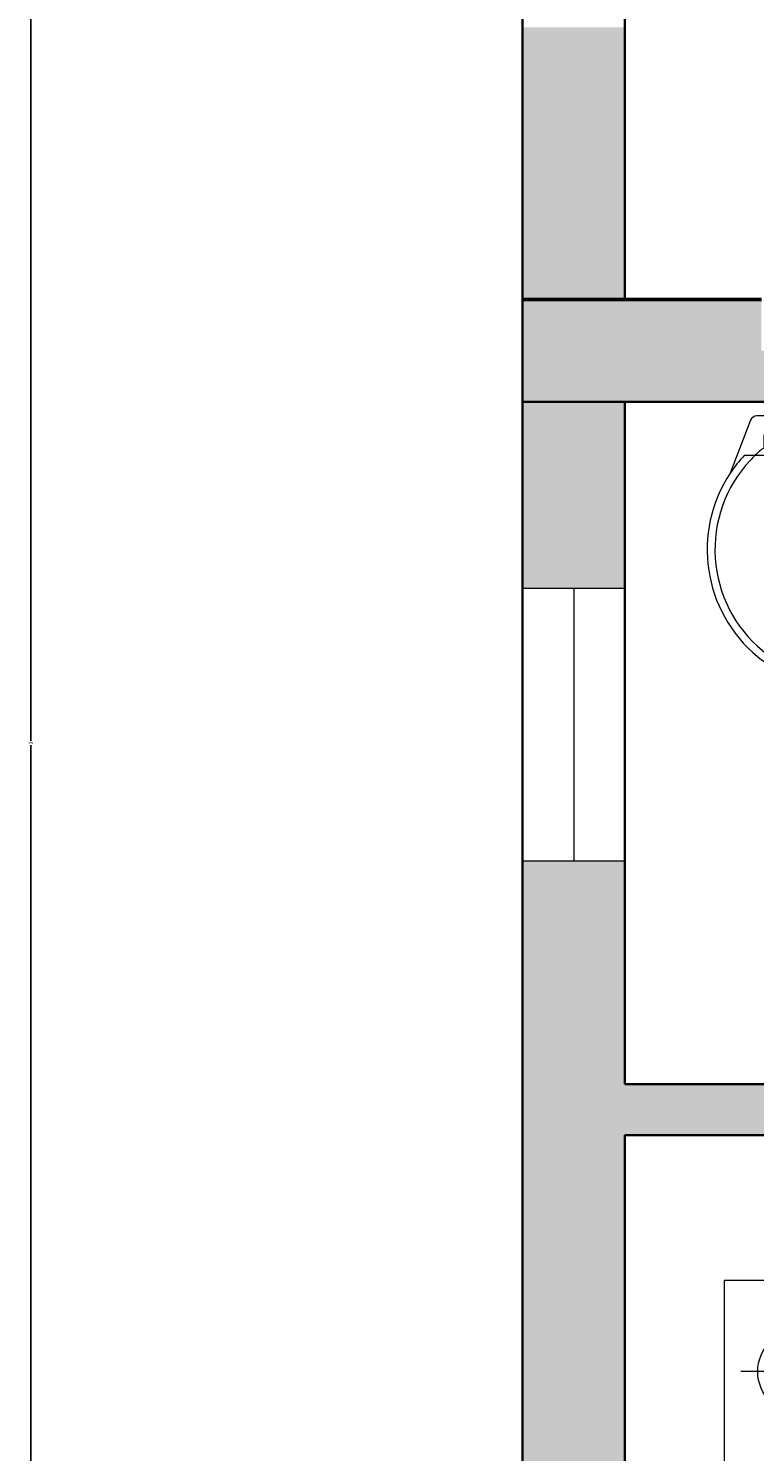
# Model space of a CAD drawing. Units: inches. Extents: x -28 to 485, y -861 to 54.
# Tile 7 of 14: x -28 to 36, y -240 to -115. Entities that reach past the tile are written whole.
import ezdxf

# ---------------------------------------------------------------- set-up
doc = ezdxf.new("R2010")
doc.units = ezdxf.units.IN
doc.header["$MEASUREMENT"] = 0
for name, color, linetype, lineweight in [('A-ANNO-DIMS', 2, 'Continuous', 18), ('A-COLS', 7, 'Continuous', 50), ('A-COLS-PATT', 8, 'Continuous', 13), ('A-FLOR-FIXT', 9, 'Continuous', 18), ('A-FURN', 8, 'Continuous', 13), ('A-GLAZ', 4, 'Continuous', 18), ('A-WALL', 7, 'Continuous', 35), ('A-WALL-PATT', 34, 'Continuous', 13)]:
    doc.layers.add(name, color=color, linetype=linetype, lineweight=lineweight)
doc.styles.get("Standard").update_dxf_attribs({"font": 'arial.ttf'})
doc.dimstyles.get("Standard").update_dxf_attribs({"dimtxt": 0.18, "dimasz": 0.18, "dimexe": 0.18, "dimexo": 0.0625, "dimgap": 0.09, "dimtad": 0, "dimtih": 1, "dimtoh": 1, "dimdec": 0, "dimzin": 0, "dimdsep": 46, "dimlunit": 3, "dimtxsty": 'Standard', "dimcen": 0.09, "dimadec": 0, "dimazin": 0, "dimtfac": 1, "dimtdec": 0, "dimtofl": 0, "dimtmove": 0, "dimatfit": 3, "dimfxl": 1, "dimtolj": 1, "dimtzin": 0, "dimarcsym": 0})

# ---------------------------------------------------------------- blocks, each defined once
blk = doc.blocks.new('BED-DOUBLE-WITH-NIGHTSTANDS')
for p, q in [((0, 0), (0, 80.08)), ((6.67, 66.84), (6.67, 77.31)), ((11.91, 72.08), (1.44, 72.08)), ((39.26, 64.51), (39.26, 68.96)), ((39.26, 68.96), (68.11, 68.96)), ((68.11, 68.96), (68.11, 10.57)), ((40.19, 68.03), (40.19, 64.5)), ((67.18, 68.03), (40.19, 68.03)), ((67.18, 11.5), (67.18, 68.03)), ((1.03, 64.07), (1.03, 16.02)), ((12.66, 16.02), (12.66, 64.07)), ((15.98, 63.85), (16.38, 35.34)), ((44.25, 64.43), (44.25, 15.09)), ((45.25, 64.51), (45.25, 15.09)), ((16.8, 63.82), (17.22, 34.74)), ((19.33, 63.78), (19.45, 33.37)), ((20.15, 63.78), (20.27, 33.06)), ((59.06, 60.14), (58.15, 60.31)), ((53.12, 56.3), (53.12, 23.78)), ((59.06, 54.54), (58.15, 54.36)), ((12.66, 38.02), (18.76, 33.63)), ((15.04, 27.14), (12.66, 35.87)), ((18.76, 33.63), (23.47, 31.84)), ((23.47, 31.84), (25.57, 31.52)), ((25.57, 31.52), (24.92, 28.93)), ((24.92, 28.93), (23.95, 26.82)), ((17.14, 21.3), (15.04, 27.14)), ((23.95, 26.82), (23.47, 23.25)), ((59.06, 24.99), (58.15, 25.16)), ((23.47, 23.25), (23.14, 19.19)), ((19.41, 18.22), (17.14, 21.3)), ((23.14, 19.19), (23.47, 15.95)), ((59.06, 19.39), (58.15, 19.21)), ((22.82, 15.3), (19.41, 18.22)), ((0, 16.02), (21.98, 16.02)), ((23.47, 15.95), (22.82, 15.3)), ((39.26, 10.57), (39.26, 15.1)), ((40.19, 15.1), (40.19, 11.5)), ((6.67, 13.24), (6.67, 2.78)), ((40.19, 11.5), (67.18, 11.5)), ((68.11, 10.57), (39.26, 10.57)), ((11.91, 8.01), (1.44, 8.01))]:
    blk.add_line(p, q)
for points in [[(0, 64.07), (13.35, 64.07), (13.35, 80.08), (0, 80.08)], [(6.67, 72.08), (5.06, 71.14)], [(6.67, 72.08), (8.29, 71.14)], [(13.35, 16.02), (13.35, 0), (0, 0)], [(6.67, 8.01), (5.06, 8.94)], [(6.67, 8.01), (8.29, 8.94)]]:
    blk.add_lwpolyline(points)
for points in [[(43.62, 64.41, 0.056112), (48.03, 64.99, 0.095341), (52.27, 66.12)], [(2, 59.47, -0.074897), (7.23, 59.37, 0.472817)], [(7.52, 43.09, -0.14099), (2.18, 42.93, -0.235245)], [(7.52, 39.67, 0.14099), (2.18, 39.83, 0.235245)], [(2, 20.62, 0.074897), (7.23, 20.71, -0.472817)], [(30.15, 15.13, 0.001242), (45.35, 15.09, -0.127202), (52.92, 13.49)]]:
    blk.add_lwpolyline(points, format="xyb")
for centre, radius in [((6.67, 72.08), 3.74), ((6.67, 72.08), 1.87), ((64.11, 56.84), 0.204), ((61.96, 55.51), 0.204), ((61.96, 24.02), 0.204), ((64.11, 22.68), 0.204), ((6.67, 8.01), 3.74), ((6.67, 8.01), 1.87)]:
    blk.add_circle(centre, radius)
for centre, radius, start, end in [((69.62, 57.92), 10.46, 111.4092, 145.6135), ((68.59, 75.81), 10.46, 228.1144, 262.255), ((69.99, 70.57), 5.1, 209.8884, 236.5383), ((70.94, 72.4), 6.35, 223.5186, 233.6964), ((52.68, 65.51), 0.73, 336.5219, 123.8264), ((131.01, 58.75), 77.93, 175.2402, 181.8035), ((22.44, 207.63), 143.9, 266.1, 270.9282), ((27.68, 251.44), 187.71, 269.1145, 274.8735), ((60.79, 62.99), 0.867, 76.272, 177.0484), ((61.24, 62.69), 1.16, 20.9613, 102.2885), ((68.81, 67.71), 4.25, 221.0454, 247.4453), ((66.52, 79.36), 14.47, 266.3481, 272.5919), ((58.76, 65.61), 6.06, 203.6453, 236.3329), ((55.85, 62.08), 1.35, 88.9462, 185.5144), ((56.04, 61.53), 1.91, 7.1143, 95.0551), ((59.12, 61.97), 1.2, 19.1312, 189.736), ((60.43, 62.21), 0.737, 126.7319, 206.0245), ((59.47, 64.76), 1.79, 284.7031, 328.6173), ((61.96, 62.49), 1.65, 125.7657, 194.5347), ((53.85, 65.41), 7.32, 332.8176, 347.4827), ((61.86, 63.85), 0.873, 181.7131, 301.5367), ((59, 62.09), 2.64, 2.0648, 41.1598), ((60.59, 63.07), 0.856, 316.2238, 62.3173), ((61.09, 62.57), 0.0682, 20.2667, 316.2271), ((56.85, 62.5), 2.41, 193.079, 274.7067), ((55.32, 60.77), 1.86, 338.5779, 68.4181), ((55.62, 61.86), 2.33, 305.9599, 357.6409), ((56.48, 64.35), 3.78, 288.2955, 328.7386), ((58.76, 62.26), 1.5, 285.6955, 4.031), ((60.76, 60.64), 1.6, 128.4175, 173.8338), ((61.51, 62.18), 0.13, 168.5166, 2.0648), ((61.45, 62.19), 0.0631, 52.0591, 168.5166), ((53.71, 63.39), 3.32, 259.249, 301.1782), ((55.15, 57.49), 3.09, 85.2696, 124.215), ((57.33, 61.13), 1.99, 196.8663, 330.0915), ((55.15, 57.49), 3.09, 53.6555, 57.2989), ((56.78, 64.39), 4.3, 273.4924, 303.7117), ((-760.15, 15.33), 763.42, 2.85022, 3.31479), ((9.33, 49.26), 10.32, 78.2417, 114.8684), ((1.06, 56.61), 10.73, 348.9631, 14.8961), ((54, 59.28), 0.964, 127.675, 162.5814), ((54, 59.28), 0.964, 196.6343, 225.5483), ((54.57, 60.82), 2.55, 240.8249, 340.7178), ((53.81, 59.69), 1.2, 246.1646, 318.4347), ((55.03, 61.2), 2.3, 240.0851, 262.564), ((55.94, 57.8), 1.64, 74.8529, 138.4347), ((56.5, 59.87), 0.497, 254.8529, 12.6959), ((60.19, 59.12), 0.158, 125.0752, 284.7644), ((60.43, 59.18), 0.34, 127.3642, 168.4363), ((60.17, 59.45), 0.49, 277.4968, 341.2737), ((60.56, 59.22), 0.195, 88.1325, 178.8919), ((60.95, 59.02), 0.422, 136.3462, 189.6513), ((60.71, 58.98), 0.176, 189.6513, 312.3208), ((60.75, 59.46), 0.204, 183.2768, 356.7232), ((61.39, 59.1), 0.668, 164.2829, 186.9148), ((60.6, 59.09), 0.334, 312.3208, 40.2111), ((61.31, 59.47), 0.474, 201.6382, 274.947), ((60.68, 58.82), 0.619, 42.3896, 66.5724), ((66.93, 63.72), 7.6, 217.9541, 226.8459), ((61.13, 59.18), 0.337, 10.9597, 52.2379), ((61.33, 59.15), 0.156, 274.947, 37.5263), ((62.33, 58.47), 0.42, 115.5379, 168.6744), ((60.9, 59.07), 1.27, 329.344, 349.7412), ((59.89, 58.78), 2.26, 352.8698, 1.6736), ((61.28, 51.56), 6.63, 110.1059, 116.9968), ((59.01, 57.53), 0.163, 83.9457, 185.6216), ((58.36, 57.69), 0.671, 328.836, 0.8141), ((58.71, 57.49), 0.384, 306.5232, 32.4668), ((59.16, 57.79), 0.163, 112.5583, 214.2343), ((59.06, 58.08), 0.384, 265.7131, 351.6568), ((58.72, 58.29), 0.671, 297.3659, 329.344), ((58.21, 58.87), 1.29, 313.6929, 321.7899), ((59.64, 57.99), 0.42, 115.5379, 168.6744), ((58.21, 58.6), 1.27, 329.344, 349.7412), ((61.28, 51.56), 6.63, 86.1723, 106.4158), ((57.2, 58.31), 2.26, 352.8698, 1.6736), ((61.86, 58.27), 0.163, 112.5583, 214.2343), ((61.75, 58.56), 0.384, 265.7131, 351.6568), ((61.42, 58.77), 0.671, 297.3659, 329.344), ((61.45, 54.86), 3.33, 60.7959, 85.244), ((54.37, 50.07), 10.94, 37.8256, 47.7588), ((60.91, 59.35), 1.29, 313.6929, 321.7899), ((63.07, 58.33), 0.228, 33.0979, 123.1364), ((58.05, 55.12), 5.96, 31.1156, 34.8118), ((62.74, 57.94), 0.617, 2.3172, 70.5201), ((62.44, 57.27), 0.93, 310.9365, 22.7695), ((63.25, 57.78), 0.178, 135.7354, 318.1297), ((62.95, 58.07), 0.236, 315.7354, 31.1156), ((62.75, 57.57), 0.547, 319.3812, 5.5456), ((63.38, 57.79), 0.178, 68.2452, 250.6395), ((62.97, 58), 0.531, 352.6008, 57.1845), ((64.87, 54.44), 3.55, 111.7087, 116.2181), ((61.45, 54.86), 3.33, 47.5083, 55.9967), ((63.48, 58.12), 0.531, 252.8042, 349.6943), ((62.97, 57.17), 0.565, 331.1838, 51.6792), ((63.53, 58.17), 0.236, 248.2452, 323.6254), ((63.33, 58.31), 0.617, 291.7087, 3.0299), ((58.93, 61.56), 5.96, 323.6254, 327.3216), ((63.81, 58.16), 0.228, 325.6077, 55.6462), ((54.57, 53.85), 2.55, 19.2822, 119.1751), ((57.16, 57.12), 0.251, 169.5864, 349.5616), ((57.25, 57.11), 0.154, 349.5616, 167.2949), ((59.06, 57.02), 0.42, 129.5056, 182.6421), ((57.85, 58), 1.27, 308.4388, 328.836), ((57.63, 59.02), 2.26, 296.5064, 305.3102), ((57.61, 57.86), 1.29, 336.3901, 344.4871), ((61.66, 57.07), 0.93, 253.6301, 325.4631), ((61.92, 55.78), 0.658, 82.0748, 142.6895), ((61.87, 56.57), 0.565, 273.8774, 357.1501), ((62.09, 56.97), 0.547, 262.0748, 308.2393), ((62.97, 56.41), 0.565, 181.4625, 249.4747), ((62.87, 56.86), 0.547, 215.1128, 261.2773), ((63.31, 56.83), 0.93, 197.889, 269.722), ((65.87, 54.52), 3.99, 130.182, 149.456), ((63.67, 56.79), 0.658, 139.3812, 199.9959), ((62.87, 57.22), 0.675, 285.6484, 332.2957), ((63.55, 56.5), 0.158, 125.0752, 284.7644), ((63.8, 56.56), 0.34, 93.635, 168.4363), ((63.75, 57.1), 0.2, 138.2946, 276.2474), ((63.53, 56.83), 0.49, 277.4968, 341.2737), ((63.83, 57.07), 0.278, 358.5719, 143.8954), ((63.92, 56.61), 0.195, 88.1325, 178.8919), ((63.99, 57.29), 0.281, 208.8493, 269.9355), ((63.75, 57.22), 0.321, 274.2123, 318.1587), ((64.31, 56.4), 0.422, 136.3462, 189.6513), ((64.75, 56.48), 0.668, 164.2829, 186.9148), ((64.73, 56.9), 0.643, 121.9501, 165.2442), ((63.96, 56.47), 0.334, 312.3208, 40.2111), ((64.67, 56.85), 0.474, 201.6382, 274.947), ((64.28, 57.14), 0.135, 262.868, 7.094), ((64.04, 56.2), 0.619, 42.3896, 66.5724), ((64.27, 57.26), 0.403, 278.5614, 22.5914), ((64.49, 56.56), 0.337, 10.9597, 118.7804), ((64.49, 57.27), 0.202, 44.3732, 121.9501), ((64.7, 56.53), 0.156, 274.947, 37.5263), ((54, 55.39), 0.964, 134.4517, 156.7144), ((53.81, 54.99), 1.2, 41.5653, 113.8354), ((55.03, 53.47), 2.3, 97.436, 119.9149), ((55.94, 56.87), 1.64, 221.5653, 285.1471), ((57.33, 53.55), 1.99, 29.9085, 163.1337), ((56.5, 54.81), 0.497, 347.3041, 105.1471), ((61.4, 55.17), 0.158, 125.0752, 284.7644), ((61.65, 55.23), 0.34, 93.635, 168.4363), ((61.85, 56.68), 0.675, 228.342, 274.9894), ((61.6, 55.76), 0.2, 138.2946, 276.2474), ((61.38, 55.5), 0.49, 277.4968, 341.2737), ((61.68, 55.73), 0.278, 358.5719, 143.8954), ((61.77, 55.27), 0.195, 88.1325, 178.8919), ((61.84, 55.95), 0.281, 208.8493, 269.9355), ((61.6, 55.89), 0.321, 274.2123, 318.1587), ((62.16, 55.06), 0.422, 136.3462, 189.6513), ((62.6, 55.14), 0.668, 164.2829, 186.9148), ((62.58, 55.56), 0.643, 121.9501, 165.2442), ((61.81, 55.14), 0.334, 312.3208, 40.2111), ((62.52, 55.52), 0.474, 201.6382, 274.947), ((62.13, 55.81), 0.135, 262.868, 7.094), ((61.89, 54.87), 0.619, 42.3896, 66.5724), ((62.12, 55.92), 0.403, 278.5614, 22.5914), ((62.34, 55.23), 0.337, 10.9597, 118.7804), ((65.87, 54.52), 3.99, 156.1523, 156.9499), ((62.34, 55.94), 0.202, 44.3732, 121.9501), ((62.55, 55.2), 0.156, 274.947, 37.5263), ((63.02, 56.51), 0.675, 248.3627, 295.0101), ((62.69, 55.67), 0.658, 20.6625, 81.2773), ((64.07, 56.36), 0.176, 189.6513, 312.3208), ((1.85, 51.98), 10.19, 333.8761, 16.1746), ((54, 55.39), 0.964, 203.2856, 232.325), ((53.71, 51.28), 3.32, 58.8218, 100.2867), ((58.76, 49.06), 6.06, 123.6671, 158.5059), ((55.15, 57.18), 3.09, 235.785, 274.7304), ((56.85, 52.18), 2.41, 85.2933, 166.921), ((55.32, 53.9), 1.86, 291.5819, 21.4221), ((55.15, 57.18), 3.09, 302.7011, 306.3445), ((55.62, 52.81), 2.33, 2.3591, 54.0401), ((56.78, 50.29), 4.3, 56.2883, 86.5076), ((56.48, 50.32), 3.78, 31.2614, 71.7045), ((60.76, 54.03), 1.6, 186.1662, 231.5825), ((58.76, 52.42), 1.5, 355.969, 74.3045), ((61.92, 55.02), 0.176, 189.6513, 312.3208), ((65.87, 54.52), 3.99, 175.2415, 182.8929), ((16.01, 49.96), 14.08, 166.3427, 191.1841), ((55.85, 52.59), 1.35, 174.4856, 271.0538), ((56.04, 53.15), 1.91, 264.9449, 352.8857), ((59.12, 52.71), 1.2, 170.264, 340.8688), ((60.43, 52.46), 0.737, 153.9755, 233.2681), ((61.96, 52.19), 1.65, 165.4653, 234.2343), ((53.85, 49.26), 7.32, 12.5173, 27.1824), ((61.51, 52.5), 0.13, 357.9352, 191.4834), ((60.79, 51.69), 0.867, 182.9516, 283.728), ((59.47, 49.92), 1.79, 31.3827, 75.2969), ((59, 52.59), 2.64, 318.8402, 357.9352), ((60.59, 51.6), 0.856, 297.6827, 43.7762), ((61.86, 50.82), 0.873, 58.4633, 178.2869), ((61.24, 51.98), 1.16, 257.7115, 339.0387), ((61.13, 52.12), 0.113, 43.7762, 339.7183), ((61.45, 52.48), 0.0631, 191.4834, 307.9409), ((69.62, 56.75), 10.46, 214.3865, 248.5908), ((68.81, 46.96), 4.25, 112.5547, 138.9546), ((66.17, 41.19), 8.09, 82.8636, 171.8197), ((66.52, 35.31), 14.47, 87.4081, 93.6519), ((66.74, 46.53), 1.88, 76.3898, 169.0739), ((74.19, 42.33), 10.46, 152.5854, 175.5377), ((66.48, 45.12), 2.37, 72.8609, 131.9049), ((65.43, 42.24), 4.68, 68.117, 96.6195), ((72.68, 45.26), 5.75, 162.9798, 196.4569), ((5.99, 44.03), 3.96, 153.3437, 196.1026), ((7.37, 44.56), 4.25, 335.0183, 18.5407), ((75.64, 42.98), 8.5, 174.3643, 175.6213), ((10.2, 52.53), 9.81, 254.1707, 275.9871), ((58.94, 41.49), 1.16, 50.8855, 132.2127), ((64.01, 42.31), 0.867, 106.1963, 206.9726), ((61.98, 43.19), 1.79, 314.6273, 358.5415), ((65.27, 42.46), 1.65, 155.6899, 224.4589), ((64.54, 42.29), 1.16, 50.8855, 132.2127), ((64.51, 43.6), 0.873, 211.6373, 331.4609), ((63.8, 42.29), 0.856, 346.148, 92.2415), ((62.91, 40.64), 2.64, 31.989, 71.0841), ((56.78, 40.96), 7.32, 2.7418, 17.407), ((81.47, 38.5), 15.2, 160.0972, 160.2783), ((58.4, 41.51), 0.867, 106.1963, 206.9726), ((56.38, 42.39), 1.79, 314.6273, 358.5415), ((59.67, 41.66), 1.65, 155.6899, 224.4589), ((59.67, 40.53), 1.65, 135.5411, 204.3101), ((58.91, 42.8), 0.873, 211.6373, 331.4609), ((58.2, 41.49), 0.856, 346.148, 92.2415), ((57.3, 39.84), 2.64, 31.989, 71.0841), ((51.18, 40.16), 7.32, 2.7418, 17.407), ((51.18, 42.04), 7.32, 342.593, 357.2582), ((58.87, 41.3), 0.0682, 50.1909, 346.0209), ((64.47, 42.1), 0.0682, 50.1909, 346.0209), ((64.98, 41.95), 0.0631, 81.9833, 198.4408), ((65.04, 41.98), 0.13, 198.4408, 31.989), ((58.4, 40.68), 0.867, 153.0274, 253.8037), ((56.38, 39.81), 1.79, 1.4585, 45.3727), ((57.3, 42.35), 2.64, 288.9159, 328.011), ((58.2, 40.71), 0.856, 267.7585, 13.852), ((58.91, 39.39), 0.873, 28.5391, 148.3627), ((58.92, 40.88), 0.113, 13.852, 309.9245), ((59.44, 41.17), 0.13, 198.4408, 31.989), ((59.37, 41.15), 0.0631, 81.9833, 198.4408), ((59.44, 41.02), 0.13, 328.011, 161.5592), ((59.37, 41.04), 0.0631, 161.5592, 278.0167), ((64.01, 39.88), 0.867, 153.0274, 253.8037), ((61.98, 39.01), 1.79, 1.4585, 45.3727), ((65.27, 39.73), 1.65, 135.5411, 204.3101), ((56.78, 41.24), 7.32, 342.593, 357.2582), ((62.91, 41.55), 2.64, 288.9159, 328.011), ((63.8, 39.91), 0.856, 267.7585, 13.852), ((64.52, 40.08), 0.113, 13.852, 309.9245), ((64.98, 40.24), 0.0631, 161.5592, 278.0167), ((65.04, 40.22), 0.13, 328.011, 161.5592), ((16.3, 37.72), 14.27, 171.5249, 193.96), ((10.2, 30.23), 9.81, 84.0129, 105.8293), ((-2.51, 36.66), 14.12, 349.8617, 13.6238), ((58.94, 40.71), 1.16, 227.7873, 309.1145), ((68.59, 40.66), 10.46, 184.4623, 262.255), ((64.51, 38.59), 0.873, 28.5391, 148.3627), ((64.54, 39.91), 1.16, 227.7873, 309.1145), ((74.19, 39.86), 10.46, 184.4623, 207.4146), ((72.68, 36.94), 5.75, 163.5431, 197.0202), ((75.64, 39.22), 8.5, 184.3787, 185.6357), ((81.47, 43.7), 15.2, 199.7217, 199.9028), ((30.98, 31.59), 29.04, 172.2196, 189.497), ((-6.57, 29.12), 18.61, 348.0397, 19.2615), ((69.99, 35.42), 5.1, 181.272, 236.5383), ((72.72, 40.59), 9.45, 214.0123, 234.053), ((70.94, 37.25), 6.35, 197.8504, 233.6964), ((-4.69, 37.08), 31.06, 340.1194, 349.3383), ((25.64, 31.34), 0.193, 358.8623, 109.7536), ((69.62, 22.77), 10.46, 111.4092, 145.6135), ((66.52, 44.21), 14.47, 266.3481, 272.5919), ((68.81, 32.56), 4.25, 221.0454, 247.4453), ((58.76, 30.46), 6.06, 201.4941, 236.3329), ((55.85, 26.93), 1.35, 88.9462, 185.5144), ((56.04, 26.38), 1.91, 7.1143, 95.0551), ((59.12, 26.82), 1.2, 19.1312, 189.736), ((60.43, 27.07), 0.737, 126.7319, 206.0245), ((60.79, 27.84), 0.867, 76.272, 177.0484), ((59.47, 29.61), 1.79, 284.7031, 328.6173), ((61.96, 27.34), 1.65, 125.7657, 194.5347), ((53.85, 30.27), 7.32, 332.8176, 347.4827), ((61.24, 27.55), 1.16, 20.9613, 102.2885), ((60.59, 27.92), 0.856, 316.2238, 62.3173), ((59, 26.94), 2.64, 2.0648, 41.1598), ((61.86, 28.71), 0.873, 181.7131, 301.5367), ((-760.15, 64.76), 763.42, 356.68521, 357.14978), ((30.48, 23.89), 6.52, 156.2616, 191.3392), ((56.85, 27.35), 2.41, 193.079, 274.7067), ((55.32, 25.63), 1.86, 338.5779, 68.4181), ((55.62, 26.71), 2.33, 305.9599, 357.6409), ((56.48, 29.2), 3.78, 288.2955, 328.7386), ((58.76, 27.11), 1.5, 285.6955, 4.031), ((60.76, 25.49), 1.6, 128.4175, 173.8338), ((61.09, 27.42), 0.0682, 20.2667, 316.2271), ((61.51, 27.03), 0.13, 168.5166, 2.0648), ((61.45, 27.04), 0.0631, 52.0591, 168.5166), ((1.06, 23.47), 10.73, 345.1039, 11.0369), ((53.71, 28.24), 3.32, 259.7133, 301.1782), ((55.15, 22.34), 3.09, 85.2696, 124.215), ((57.33, 25.98), 1.99, 196.8663, 330.0915), ((56.78, 29.24), 4.3, 273.4924, 303.7117), ((65.87, 25.01), 3.99, 177.1071, 184.7585), ((136.48, 22.83), 83.37, 179.3433, 185.6887), ((54, 24.13), 0.964, 127.675, 156.7144), ((54.57, 25.67), 2.55, 240.8249, 340.7178), ((55.03, 26.06), 2.3, 240.0851, 262.564), ((55.94, 22.65), 1.64, 74.8529, 138.4347), ((56.5, 24.72), 0.497, 254.8529, 12.6959), ((55.15, 22.34), 3.09, 53.6555, 57.2989), ((61.4, 24.36), 0.158, 75.2356, 234.9248), ((61.65, 24.3), 0.34, 191.5637, 266.365), ((61.6, 23.76), 0.2, 83.7526, 221.7054), ((61.38, 24.03), 0.49, 18.7263, 82.5032), ((61.68, 23.79), 0.278, 216.1046, 1.4281), ((61.77, 24.25), 0.195, 181.1081, 271.8675), ((61.84, 23.57), 0.281, 90.0645, 151.1507), ((61.6, 23.64), 0.321, 41.8413, 85.7877), ((61.92, 24.5), 0.176, 47.6792, 170.3487), ((62.16, 24.46), 0.422, 170.3487, 223.6538), ((62.6, 24.38), 0.668, 173.0852, 195.7171), ((62.58, 23.96), 0.643, 194.7558, 238.0499), ((61.81, 24.39), 0.334, 319.7889, 47.6792), ((62.52, 24.01), 0.474, 85.053, 158.3618), ((62.13, 23.71), 0.135, 352.906, 97.132), ((61.89, 24.66), 0.619, 293.4276, 317.6104), ((62.34, 24.29), 0.337, 241.2196, 349.0403), ((62.12, 23.6), 0.403, 337.4086, 81.4386), ((62.55, 24.33), 0.156, 322.4737, 85.053), ((-5.54, 16.67), 30.23, 357.4519, 11.3392), ((54, 24.13), 0.964, 203.229, 225.5483), ((53.81, 24.54), 1.2, 246.1646, 318.4347), ((57.16, 22.4), 0.251, 10.4384, 190.4136), ((61.85, 22.84), 0.675, 85.0106, 131.658), ((61.66, 22.46), 0.93, 34.5369, 106.3699), ((61.92, 23.75), 0.658, 217.3105, 277.9252), ((54.37, 29.45), 10.94, 312.2412, 322.1744), ((61.87, 22.95), 0.565, 2.8499, 86.1226), ((62.09, 22.55), 0.547, 51.7607, 97.9252), ((65.87, 25.01), 3.99, 203.0501, 203.8477), ((62.34, 23.59), 0.202, 238.0499, 315.6268), ((62.97, 23.11), 0.565, 110.5253, 178.5375), ((63.31, 22.7), 0.93, 90.278, 162.111), ((62.87, 22.67), 0.547, 98.7227, 144.8872), ((65.87, 25.01), 3.99, 210.544, 229.818), ((63.02, 23.01), 0.675, 64.9899, 111.6373), ((62.69, 23.86), 0.658, 278.7227, 339.3375), ((63.67, 22.74), 0.658, 160.0041, 220.6188), ((62.44, 22.26), 0.93, 337.2305, 49.0635), ((62.87, 22.31), 0.675, 27.7043, 74.3516), ((62.97, 22.35), 0.565, 308.3208, 28.8162), ((63.55, 23.03), 0.158, 75.2356, 234.9248), ((63.8, 22.96), 0.34, 191.5637, 266.365), ((63.75, 22.43), 0.2, 83.7526, 221.7054), ((63.53, 22.69), 0.49, 18.7263, 82.5032), ((63.92, 22.92), 0.195, 181.1081, 271.8675), ((63.75, 22.31), 0.321, 41.8413, 85.7877), ((64.07, 23.17), 0.176, 47.6792, 170.3487), ((64.31, 23.13), 0.422, 170.3487, 223.6538), ((64.75, 23.05), 0.668, 173.0852, 195.7171), ((63.96, 23.05), 0.334, 319.7889, 47.6792), ((64.67, 22.68), 0.474, 85.053, 158.3618), ((64.04, 23.32), 0.619, 293.4276, 317.6104), ((64.49, 22.96), 0.337, 241.2196, 349.0403), ((64.27, 22.27), 0.403, 337.4086, 81.4386), ((64.7, 22.99), 0.156, 322.4737, 85.053), ((9.33, 30.82), 10.32, 245.1316, 281.7583), ((57.25, 22.42), 0.154, 192.7051, 10.4384), ((61.28, 27.97), 6.63, 243.0032, 249.8941), ((57.85, 21.53), 1.27, 31.164, 51.5612), ((59.06, 22.5), 0.42, 177.3579, 230.4944), ((57.63, 20.5), 2.26, 54.6898, 63.4936), ((57.61, 21.66), 1.29, 15.5129, 23.6099), ((59.01, 21.99), 0.163, 174.3784, 276.0543), ((58.71, 22.03), 0.384, 327.5332, 53.4768), ((58.36, 21.84), 0.671, 359.1859, 31.164), ((59.16, 21.74), 0.163, 145.7657, 247.4417), ((59.06, 21.45), 0.384, 8.3432, 94.2869), ((58.72, 21.23), 0.671, 30.656, 62.6341), ((58.21, 20.66), 1.29, 38.2101, 46.3071), ((59.64, 21.53), 0.42, 191.3256, 244.4621), ((58.21, 20.93), 1.27, 10.2588, 30.656), ((61.28, 27.97), 6.63, 253.5842, 273.8277), ((57.2, 21.22), 2.26, 358.3264, 7.1302), ((66.93, 15.8), 7.6, 133.1541, 142.0459), ((61.86, 21.26), 0.163, 145.7657, 247.4417), ((61.45, 24.67), 3.33, 274.756, 299.2041), ((61.75, 20.97), 0.384, 8.3432, 94.2869), ((61.42, 20.76), 0.671, 30.656, 62.6341), ((62.74, 21.59), 0.617, 289.4799, 357.6828), ((58.05, 24.41), 5.96, 325.1882, 328.8844), ((63.25, 21.74), 0.178, 41.8703, 224.2646), ((62.95, 21.45), 0.236, 328.8844, 44.2646), ((62.75, 21.95), 0.547, 354.4544, 40.6188), ((63.38, 21.74), 0.178, 109.3605, 291.7548), ((62.97, 21.52), 0.531, 302.8155, 7.3992), ((64.87, 25.09), 3.55, 243.7819, 248.2913), ((61.45, 24.67), 3.33, 304.0033, 312.4917), ((63.48, 21.4), 0.531, 10.3057, 107.1958), ((63.53, 21.36), 0.236, 36.3746, 111.7548), ((63.33, 21.21), 0.617, 356.9701, 68.2913), ((63.83, 22.46), 0.278, 216.1046, 1.4281), ((58.93, 17.96), 5.96, 32.6784, 36.3746), ((63.99, 22.24), 0.281, 90.0645, 151.1507), ((63.81, 21.37), 0.228, 304.3538, 34.3923), ((64.73, 22.63), 0.643, 194.7558, 238.0499), ((64.28, 22.38), 0.135, 352.906, 97.132), ((64.49, 22.25), 0.202, 238.0499, 315.6268), ((54, 20.25), 0.964, 134.4517, 153.558), ((54.57, 18.71), 2.55, 19.2822, 119.1751), ((53.81, 19.84), 1.2, 41.5653, 113.8354), ((55.03, 18.32), 2.3, 97.436, 119.9149), ((55.94, 21.72), 1.64, 221.5653, 285.1471), ((57.33, 18.4), 1.99, 29.9085, 163.1337), ((56.5, 19.66), 0.497, 347.3041, 105.1471), ((60.19, 20.41), 0.158, 75.2356, 234.9248), ((60.43, 20.35), 0.34, 191.5637, 232.6358), ((60.17, 20.07), 0.49, 18.7263, 82.5032), ((60.56, 20.3), 0.195, 181.1081, 271.8675), ((60.71, 20.55), 0.176, 47.6792, 170.3487), ((60.95, 20.51), 0.422, 170.3487, 223.6538), ((60.75, 20.06), 0.204, 3.2768, 176.7232), ((61.39, 20.43), 0.668, 173.0852, 195.7171), ((60.6, 20.43), 0.334, 319.7889, 47.6792), ((61.31, 20.06), 0.474, 85.053, 158.3618), ((60.68, 20.7), 0.619, 293.4276, 317.6104), ((61.13, 20.34), 0.337, 307.7621, 349.0403), ((61.33, 20.37), 0.156, 322.4737, 85.053), ((60.91, 20.18), 1.29, 38.2101, 46.3071), ((62.33, 21.06), 0.42, 191.3256, 244.4621), ((60.9, 20.45), 1.27, 10.2588, 30.656), ((59.89, 20.74), 2.26, 358.3264, 7.1302), ((63.07, 21.2), 0.228, 236.8636, 326.9021), ((54, 20.25), 0.964, 210.0293, 232.325), ((53.71, 16.14), 3.32, 58.8218, 99.1554), ((58.76, 13.91), 6.06, 123.6671, 153.2997), ((55.15, 22.04), 3.09, 235.785, 274.7304), ((56.85, 17.03), 2.41, 85.2933, 166.921), ((55.32, 18.75), 1.86, 291.5819, 21.4221), ((55.15, 22.04), 3.09, 302.7011, 306.3445), ((55.62, 17.67), 2.33, 2.3591, 54.0401), ((56.78, 15.14), 4.3, 56.2883, 86.5076), ((55.85, 17.44), 1.35, 174.4856, 271.0538), ((56.04, 18), 1.91, 264.9449, 352.8857), ((56.48, 15.18), 3.78, 31.2614, 71.7045), ((59.12, 17.56), 1.2, 170.264, 340.8688), ((58.76, 17.27), 1.5, 355.969, 74.3045), ((60.76, 18.89), 1.6, 186.1662, 231.5825), ((60.43, 17.31), 0.737, 153.9755, 233.2681), ((59.47, 14.77), 1.79, 31.3827, 75.2969), ((60.79, 16.54), 0.867, 182.9516, 283.728), ((61.96, 17.04), 1.65, 165.4653, 234.2343), ((53.85, 14.11), 7.32, 12.5173, 27.1824), ((59, 17.44), 2.64, 318.8402, 357.9352), ((60.59, 16.46), 0.856, 297.6827, 43.7762), ((61.86, 15.67), 0.873, 58.4633, 178.2869), ((61.24, 16.83), 1.16, 257.7115, 339.0387), ((61.13, 16.97), 0.113, 43.7762, 339.7183), ((61.51, 17.35), 0.13, 357.9352, 191.4834), ((61.45, 17.33), 0.0631, 191.4834, 307.9409), ((24.81, -58.13), 73.46, 85.8294, 91.553), ((69.62, 21.6), 10.46, 214.3865, 248.5908), ((68.81, 11.81), 4.25, 112.5547, 138.9546), ((52.87, 14.23), 0.739, 273.98, 27.3412), ((68.59, 3.71), 10.46, 97.745, 131.8856), ((66.52, 0.17), 14.47, 87.4081, 93.6519), ((69.99, 8.96), 5.1, 123.4617, 150.1116), ((70.94, 7.13), 6.35, 126.3036, 136.4814)]:
    blk.add_arc(centre, radius, start, end)
blk = doc.blocks.new('WC-FLOOR-MOUNTED')
for p, q in [((3.27, 19.35), (4.23, 19.35)), ((4.23, 19.35), (8.71, 19.35)), ((13.2, 19.35), (8.71, 19.35)), ((13.2, 19.35), (14.16, 19.35))]:
    blk.add_line(p, q)
for points in [[(8.71, 22.81), (4.36, 22.81, 0.31031), (3.82, 22.44), (2.03, 17.79, 0.209071)], [(8.71, 22.81), (13.07, 22.81, -0.31031), (13.6, 22.44), (15.39, 17.79, -0.209071)], [(5.01, 20.04), (5.01, 21, -1), (6.47, 21), (6.47, 20.5)], [(12.41, 20.04), (12.41, 21, 1), (10.96, 21), (10.96, 20.5)], [(5.01, 20.04, 0.022712), (4.23, 19.35, 0.162618)], [(8.71, 20.04), (5.01, 20.04, 0.022712)], [(8.71, 20.04), (12.41, 20.04, -0.476108)], [(12.41, 20.04, -0.022712), (13.2, 19.35, -0.162618)], [(3.77, 18.89, 0.431639), (4.86, 2.17, 0.162618), (8.71, 0.68, 0.470877)], [(3.27, 19.35, 0.040937), (2.03, 17.79, 0.163732)], [(4.23, 19.35, 0.014165), (3.77, 18.89, 0.162618)], [(13.2, 19.35, -0.448546), (12.57, 2.17, -0.162618), (8.71, 0.68, -0.470877)], [(14.16, 19.35, -0.040937), (15.39, 17.79, -0.163732)], [(2.03, 17.79, 0.383919), (4.43, 1.64, 0.163732), (8.71, 0, 0.359733)], [(15.39, 17.79, -0.383919), (13, 1.64, -0.163732), (8.71, 0, -0.359733)]]:
    blk.add_lwpolyline(points, format="xyb")
for points in [[(10.96, 20.5), (6.47, 20.5)], [(6.47, 20.5), (6.47, 20.04)], [(10.96, 20.5), (10.96, 20.04)]]:
    blk.add_lwpolyline(points)
blk = doc.blocks.new('WINDOW-24IN')
for p, q in [((0, 24), (0, 0)), ((9, 24), (0, 24)), ((4.5, 24), (4.5, 0)), ((9, 0), (9, 24)), ((9, 0), (0, 0))]:
    blk.add_line(p, q)
blk = doc.blocks.new('*D54')
at = {"layer": 'A-ANNO-DIMS', "color": 0, "lineweight": -2, "transparency": 16777216}
for p, q in [((15.22, 10.13), (-28.15, 10.13)), ((-27.97, 9.95), (-27.97, -177.18)), ((-27.97, -364.69), (-27.97, -177.55)), ((15.22, -364.87), (-28.15, -364.87))]:
    blk.add_line(p, q, dxfattribs=at)
at = {"layer": 'A-ANNO-DIMS', "color": 0, "transparency": 16777216}
for points in [[(-28, 9.95), (-27.94, 9.95), (-27.97, 10.13)], [(-28, -364.69), (-27.94, -364.69), (-27.97, -364.87)]]:
    blk.add_solid(points, dxfattribs=at)
at = {"layer": 'Defpoints', "color": 0, "transparency": 16777216}
for p in [(15.28, 10.13), (-27.97, -364.87), (15.28, -364.87)]:
    blk.add_point(p, dxfattribs=at)
at = {"layer": 'A-ANNO-DIMS', "color": 0, "transparency": 16777216, "insert": (-27.97, -177.37), "char_height": 0.18, "attachment_point": 5}
blk.add_mtext('\\A1;375', dxfattribs=at)

msp = doc.modelspace()

# ---------------------------------------------------------------- hatches: boundary and pattern name
at = {"layer": 'A-COLS-PATT'}
h = msp.add_hatch(color=256, dxfattribs=at)
h.dxf.hatch_style = 1
h.paths.add_polyline_path([(36.285, 10.133), (15.285, 10.133), (15.285, 1.133), (36.285, 1.133)])
h.paths.add_polyline_path([(160.785, 10.133), (139.785, 10.133), (139.785, 1.133), (160.785, 1.133)])
h.paths.add_polyline_path([(316.785, 10.133), (295.785, 10.133), (295.785, 1.133), (316.785, 1.133)])
h.paths.add_polyline_path([(441.285, 10.133), (420.285, 10.133), (420.285, 1.133), (441.285, 1.133)])
h.paths.add_polyline_path([(441.285, -138.367), (432.285, -138.367), (420.285, -138.367), (420.285, -147.367), (441.285, -147.367)])
h.paths.add_polyline_path([(304.785, -130.867), (295.785, -130.867), (295.785, -147.367), (304.785, -147.367), (304.785, -142.867)])
h.paths.add_polyline_path([(160.785, -130.867), (151.785, -130.867), (151.785, -142.867), (151.785, -147.367), (160.785, -147.367)])
h.paths.add_polyline_path([(36.285, -138.367), (24.285, -138.367), (15.285, -138.367), (15.285, -147.367), (36.285, -147.367)])
h.paths.add_polyline_path([(36.285, -355.867), (15.285, -355.867), (15.285, -364.867), (36.285, -364.867)])
h.paths.add_polyline_path([(160.785, -355.867), (139.785, -355.867), (139.785, -364.867), (160.785, -364.867)])
h.paths.add_polyline_path([(316.785, -355.867), (300.285, -355.867), (295.785, -355.867), (295.785, -364.867), (316.785, -364.867)])
at = {"layer": 'A-WALL-PATT'}
h = msp.add_hatch(color=256, dxfattribs=at)
h.dxf.hatch_style = 1
h.paths.add_polyline_path([(160.785, -808.867), (160.785, -817.867), (295.785, -817.867), (295.785, -808.867)])
h.paths.add_polyline_path([(316.785, -817.867), (323.776, -817.867), (323.776, -808.867), (316.785, -808.867)])
h.paths.add_polyline_path([(420.285, -817.867), (420.285, -808.867), (383.776, -808.867), (383.776, -817.867)])
h.paths.add_polyline_path([(432.285, -808.867), (441.285, -808.867), (441.285, -702.966), (432.285, -702.966), (432.285, -708.367), (397.785, -708.367), (397.785, -710.617), (397.785, -712.867), (432.285, -712.867)])
h.paths.add_polyline_path([(300.285, -712.867), (329.285, -712.867), (329.285, -710.617), (329.285, -708.367), (295.785, -708.367), (295.785, -808.867), (300.285, -808.867)])
h.paths.add_polyline_path([(160.785, -698.867), (158.535, -698.867), (156.285, -698.867), (156.285, -808.867), (160.785, -808.867)])
h.paths.add_polyline_path([(36.285, -808.867), (36.285, -817.867), (79.721, -817.867), (79.721, -808.867)])
h.paths.add_polyline_path([(15.285, -808.867), (24.285, -808.867), (24.285, -739.09), (15.285, -739.09)])
h.paths.add_polyline_path([(24.285, -640.781), (15.285, -640.781), (15.285, -679.09), (24.285, -679.09), (24.285, -664.867), (89.285, -664.867), (89.285, -662.617), (89.285, -660.367), (24.285, -660.367)])
h.paths.add_polyline_path([(15.285, -616.781), (24.285, -616.781), (24.285, -600.367), (15.285, -600.367)])
h.paths.add_polyline_path([(36.285, -595.867), (36.285, -600.367), (123.285, -600.367), (123.285, -660.367), (117.285, -660.367), (117.285, -664.867), (156.285, -664.867), (156.285, -670.867), (160.785, -670.867), (160.785, -660.367), (127.785, -660.367), (127.785, -600.367), (129.785, -600.367), (129.785, -598.117), (129.785, -595.867)])
h.paths.add_polyline_path([(367.785, -664.867), (363.285, -664.867), (363.285, -708.367), (357.285, -708.367), (357.285, -712.867), (369.785, -712.867), (369.785, -708.367), (367.785, -708.367)])
h.paths.add_polyline_path([(432.285, -664.867), (432.285, -666.966), (441.285, -666.966), (441.285, -642.367), (432.285, -642.367), (432.285, -660.367), (328.785, -660.367), (328.785, -664.867), (363.285, -664.867)])
h.paths.add_polyline_path([(333.285, -600.367), (420.285, -600.367), (420.285, -595.867), (326.785, -595.867), (326.785, -600.367), (328.785, -600.367), (328.785, -630.367), (331.035, -630.367), (333.285, -630.367)])
h.paths.add_polyline_path([(441.285, -600.367), (432.285, -600.367), (432.285, -618.367), (441.285, -618.367)])
h.paths.add_polyline_path([(432.285, -591.367), (441.285, -591.367), (441.285, -547.793), (432.285, -547.793)])
h.paths.add_polyline_path([(295.785, -588.367), (300.238, -588.367), (300.285, -583.867), (300.285, -451.867), (295.785, -451.867)])
h.paths.add_polyline_path([(420.285, -451.867), (420.285, -442.867), (316.785, -442.867), (316.785, -451.867)])
h.paths.add_polyline_path([(432.285, -487.793), (441.285, -487.793), (441.285, -451.867), (432.285, -451.867)])
h.paths.add_polyline_path([(432.285, -442.867), (441.285, -442.867), (441.285, -364.867), (432.285, -364.867)])
h.paths.add_polyline_path([(261.785, -451.867), (261.785, -447.367), (261.785, -444.758), (261.785, -442.867), (160.785, -442.867), (160.785, -451.867)])
h.paths.add_polyline_path([(139.785, -451.867), (139.785, -442.867), (36.285, -442.867), (36.285, -451.867)])
h.paths.add_polyline_path([(15.285, -491.617), (24.285, -491.617), (24.285, -451.867), (15.285, -451.867)])
h.paths.add_polyline_path([(24.285, -551.617), (15.285, -551.617), (15.285, -591.367), (24.285, -591.367)])
h.paths.add_polyline_path([(160.785, -451.867), (156.285, -451.867), (156.285, -588.367), (160.785, -588.367)])
h.paths.add_polyline_path([(139.785, -364.867), (139.785, -355.867), (36.285, -355.867), (36.285, -364.867)])
h.paths.add_polyline_path([(24.285, -364.867), (15.285, -364.867), (15.285, -373.867), (24.285, -373.867)])
h.paths.add_polyline_path([(15.285, -433.867), (15.285, -442.867), (24.285, -442.867), (24.285, -433.867)])
h.paths.add_polyline_path([(261.785, -364.867), (261.785, -360.367), (261.785, -355.867), (160.785, -355.867), (160.785, -364.867)])
h.paths.add_polyline_path([(295.785, -355.867), (289.785, -355.867), (289.785, -364.867), (295.785, -364.867)])
h.paths.add_polyline_path([(295.785, -355.867), (300.285, -355.867), (300.285, -259.867), (333.285, -259.867), (333.285, -257.617), (333.285, -255.367), (300.285, -255.367), (300.285, -207.367), (295.785, -207.367)])
h.paths.add_polyline_path([(420.285, -364.867), (420.285, -355.867), (316.785, -355.867), (316.785, -364.867)])
h.paths.add_polyline_path([(24.285, -311.192), (15.285, -311.192), (15.285, -355.867), (24.285, -355.867)])
h.paths.add_polyline_path([(24.285, -211.867), (54.144, -211.867), (54.144, -207.367), (24.285, -207.367), (24.285, -187.772), (15.285, -187.772), (15.285, -251.192), (24.285, -251.192)])
h.paths.add_polyline_path([(82.144, -207.367), (82.144, -209.617), (82.144, -211.867), (127.785, -211.867), (127.785, -147.367), (129.785, -147.367), (129.785, -145.117), (129.785, -142.867), (36.285, -142.867), (36.285, -147.367), (123.285, -147.367), (123.285, -207.367)])
h.paths.add_polyline_path([(160.785, -207.367), (156.285, -207.367), (156.285, -355.867), (160.785, -355.867)])
h.paths.add_polyline_path([(24.285, 1.133), (15.285, 1.133), (15.285, -54.408), (24.285, -54.408)])
h.paths.add_polyline_path([(36.285, 10.133), (36.285, 1.133), (70.235, 1.133), (70.235, 10.133)])
h.paths.add_polyline_path([(15.285, -138.367), (24.285, -138.367), (24.285, -114.408), (15.285, -114.408)])
h.paths.add_polyline_path([(24.285, -147.367), (15.285, -147.367), (15.285, -163.772), (24.285, -163.772)])
h.paths.add_polyline_path([(156.285, -130.867), (160.785, -130.867), (160.785, 1.133), (156.285, 1.133)])
h.paths.add_polyline_path([(130.235, 1.133), (139.785, 1.133), (139.785, 10.133), (130.235, 10.133)])
h.paths.add_polyline_path([(316.785, 10.133), (316.785, 1.133), (328.097, 1.133), (328.097, 10.133)])
h.paths.add_polyline_path([(300.285, 1.133), (295.785, 1.133), (295.785, -130.867), (300.285, -130.867)])
h.paths.add_polyline_path([(420.285, -147.367), (420.285, -142.867), (326.785, -142.867), (326.785, -145.117), (326.785, -147.367), (328.785, -147.367), (328.785, -177.367), (331.035, -177.367), (333.285, -177.367), (333.285, -147.367)])
h.paths.add_polyline_path([(333.285, -207.367), (333.285, -205.367), (328.785, -205.367), (328.785, -211.867), (363.285, -211.867), (363.285, -255.367), (361.285, -255.367), (361.285, -259.867), (369.785, -259.867), (369.785, -255.367), (367.785, -255.367), (367.785, -211.867), (432.285, -211.867), (432.285, -214.893), (441.285, -214.893), (441.285, -188.008), (432.285, -188.008), (432.285, -207.367)])
h.paths.add_polyline_path([(441.285, -250.893), (432.285, -250.893), (432.285, -255.367), (397.785, -255.367), (397.785, -257.617), (397.785, -259.867), (432.285, -259.867), (432.285, -355.867), (441.285, -355.867)])
h.paths.add_polyline_path([(432.285, -138.367), (441.285, -138.367), (441.285, -115.099), (432.285, -115.099)])
h.paths.add_polyline_path([(441.285, -147.367), (432.285, -147.367), (432.285, -164.008), (441.285, -164.008)])
h.paths.add_polyline_path([(420.285, 1.133), (420.285, 10.133), (388.097, 10.133), (388.097, 1.133)])
h.paths.add_polyline_path([(432.285, -55.099), (441.285, -55.099), (441.285, 1.133), (432.285, 1.133)])

# ---------------------------------------------------------------- linework, layer by layer
at = {"layer": 'A-COLS'}
for p, q in [((15.285, -138.367), (24.285, -138.367)), ((24.285, -138.367), (36.285, -138.367))]:
    msp.add_line(p, q, dxfattribs=at)
at = {"layer": 'A-WALL'}
for p, q in [((15.285, 10.133), (15.285, -817.867)), ((24.285, 1.133), (24.285, -138.367)), ((15.285, -147.367), (123.285, -147.367)), ((24.285, -147.367), (24.285, -207.367)), ((24.285, -207.367), (123.285, -207.367)), ((24.285, -211.867), (127.785, -211.867)), ((24.285, -211.867), (24.285, -355.867))]:
    msp.add_line(p, q, dxfattribs=at)

# ---------------------------------------------------------------- block references
at = {"layer": 'A-FLOR-FIXT'}
msp.add_blockref('WC-FLOOR-MOUNTED', (31.516, -171.414), dxfattribs=at)
at = {"layer": 'A-FURN'}
msp.add_blockref('BED-DOUBLE-WITH-NIGHTSTANDS', (33.033, -304.743), dxfattribs=at)
at = {"layer": 'A-GLAZ'}
msp.add_blockref('WINDOW-24IN', (15.285, -187.772), dxfattribs=at)

# ---------------------------------------------------------------- dimensions: what is measured, and where the dimension line sits
at = {"layer": 'A-ANNO-DIMS'}
dim = msp.add_linear_dim(base=(-27.965, -364.867), p1=(15.285, 10.133), p2=(15.285, -364.867), angle=90, dimstyle='Standard', override={"dimdec": 0, "dimlfac": 1, "dimrnd": 0, "dimzin": 0, "dimdsep": 46, "dimlunit": 2}, dxfattribs=at)
dim.commit()
dim.dimension.update_dxf_attribs({"geometry": '*D54', "text_midpoint": (-27.965, -177.367)})

doc.saveas('drawing.dxf')
